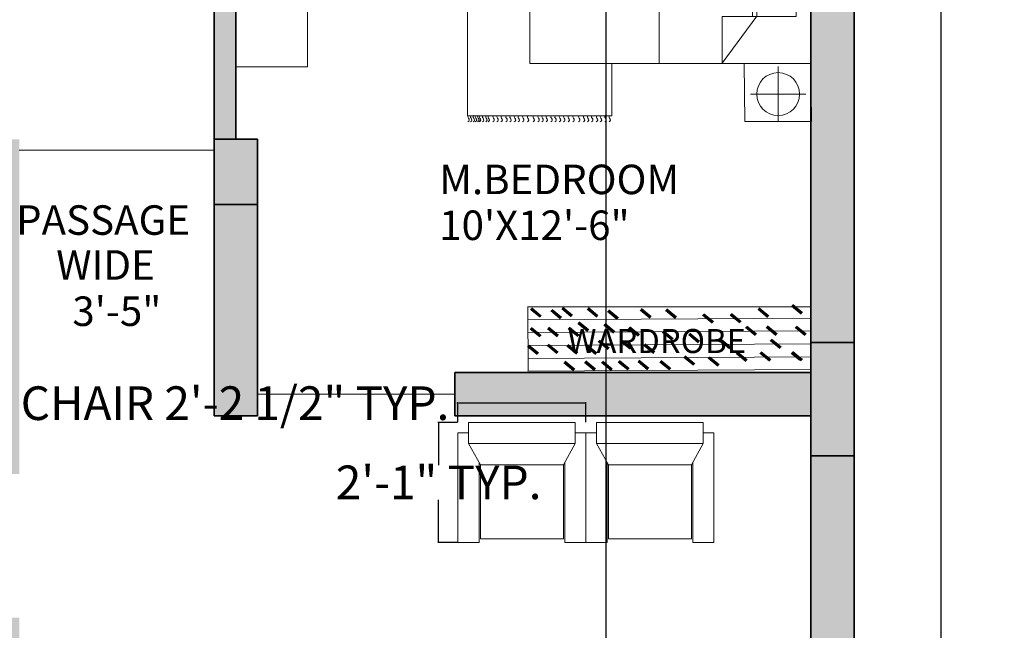
# Model space of a CAD drawing. Units: inches. Extents: x -17 to 892, y -721 to 172.
# Tile 5 of 11: x 174 to 378, y -209 to -82. Entities that reach past the tile are written whole.
import ezdxf

# ---------------------------------------------------------------- set-up
doc = ezdxf.new("R2010")
doc.units = ezdxf.units.IN
doc.header["$MEASUREMENT"] = 0
doc.layers.get('0').update_dxf_attribs({"color": 14})
for name, color, linetype, lineweight in [('A-ANNO-DIMS', 2, 'Continuous', 18), ('A-ANNO-TEXT', 7, 'Continuous', 18), ('A-AREA-IDEN', 7, 'Continuous', 18), ('A-COLS', 252, 'Continuous', 35), ('A-FLOR-CASE', 252, 'Continuous', 18), ('A-FURN-PATT', 252, 'Continuous', 9), ('A-WALL-PATT', 14, 'Continuous', 13), ('doors', 4, 'Continuous', 18), ('furniture', 252, 'Continuous', 18), ('walls', 252, 'Continuous', 35)]:
    doc.layers.add(name, color=color, linetype=linetype, lineweight=lineweight)
doc.layers.add('A-COLS-PATT', color=254, linetype='Continuous', lineweight=13, true_color=0xd7ebd2)
doc.styles.get("Standard").update_dxf_attribs({"font": 'arial.ttf'})
doc.dimstyles.get("Standard").update_dxf_attribs({"dimtxt": 7, "dimasz": 0.18, "dimexe": 0.18, "dimexo": 0.0625, "dimgap": 0.09, "dimtad": 0, "dimtih": 1, "dimtoh": 1, "dimzin": 0, "dimdsep": 46, "dimlunit": 3, "dimtxsty": 'Standard', "dimcen": 0.09, "dimadec": 0, "dimazin": 0, "dimtfac": 1, "dimtofl": 0, "dimtmove": 0, "dimatfit": 3, "dimfxl": 1, "dimtolj": 1, "dimtzin": 0, "dimarcsym": 0})

# ---------------------------------------------------------------- blocks, each defined once
blk = doc.blocks.new('CARPET')
at = {"layer": 'furniture'}
for p, q in [((-51.53, -98.11), (-51.53, -55.12)), ((-51.53, -55.12), (-41.27, -55.12)), ((36, -55.12), (51.55, -55.12)), ((51.55, -55.12), (51.55, -98.11)), ((51.55, -98.11), (-51.53, -98.11))]:
    blk.add_line(p, q, dxfattribs=at)
for points, knots in [([(-53.37, -55.99), (-53.22, -55.8), (-52.9, -55.41), (-52.34, -55.8), (-51.89, -56.08), (-51.65, -55.91), (-51.53, -55.83)], [0, 0, 0, 0, 0.653278, 1.290138, 1.740457, 2.114451, 2.114451, 2.114451, 2.114451]), ([(53.37, -55.99), (53.22, -55.8), (52.9, -55.41), (52.34, -55.8), (51.89, -56.08), (51.65, -55.91), (51.53, -55.83)], [0, 0, 0, 0, 0.653278, 1.290138, 1.740457, 2.114451, 2.114451, 2.114451, 2.114451]), ([(-53.37, -57.26), (-53.22, -57.07), (-52.9, -56.67), (-52.34, -57.07), (-51.89, -57.35), (-51.65, -57.17), (-51.53, -57.1)], [0, 0, 0, 0, 0.653278, 1.290138, 1.740457, 2.114451, 2.114451, 2.114451, 2.114451]), ([(-53.37, -58.59), (-53.22, -58.4), (-52.9, -58.01), (-52.34, -58.4), (-51.89, -58.68), (-51.65, -58.5), (-51.53, -58.43)], [0, 0, 0, 0, 0.653278, 1.290138, 1.740457, 2.114451, 2.114451, 2.114451, 2.114451]), ([(53.37, -57.26), (53.22, -57.07), (52.9, -56.67), (52.34, -57.07), (51.89, -57.35), (51.65, -57.17), (51.53, -57.1)], [0, 0, 0, 0, 0.653278, 1.290138, 1.740457, 2.114451, 2.114451, 2.114451, 2.114451]), ([(53.37, -58.59), (53.22, -58.4), (52.9, -58.01), (52.34, -58.4), (51.89, -58.68), (51.65, -58.5), (51.53, -58.43)], [0, 0, 0, 0, 0.653278, 1.290138, 1.740457, 2.114451, 2.114451, 2.114451, 2.114451]), ([(-53.37, -59.78), (-53.22, -59.58), (-52.9, -59.19), (-52.34, -59.58), (-51.89, -59.86), (-51.65, -59.69), (-51.53, -59.61)], [0, 0, 0, 0, 0.653278, 1.290138, 1.740457, 2.114451, 2.114451, 2.114451, 2.114451]), ([(-53.37, -61.22), (-53.22, -61.02), (-52.9, -60.63), (-52.34, -61.02), (-51.89, -61.3), (-51.65, -61.13), (-51.53, -61.05)], [0, 0, 0, 0, 0.653278, 1.290138, 1.740457, 2.114451, 2.114451, 2.114451, 2.114451]), ([(53.37, -59.78), (53.22, -59.58), (52.9, -59.19), (52.34, -59.58), (51.89, -59.86), (51.65, -59.69), (51.53, -59.61)], [0, 0, 0, 0, 0.653278, 1.290138, 1.740457, 2.114451, 2.114451, 2.114451, 2.114451]), ([(53.37, -61.22), (53.22, -61.02), (52.9, -60.63), (52.34, -61.02), (51.89, -61.3), (51.65, -61.13), (51.53, -61.05)], [0, 0, 0, 0, 0.653278, 1.290138, 1.740457, 2.114451, 2.114451, 2.114451, 2.114451]), ([(-53.37, -62.44), (-53.22, -62.25), (-52.9, -61.86), (-52.34, -62.25), (-51.89, -62.53), (-51.65, -62.36), (-51.53, -62.28)], [0, 0, 0, 0, 0.653278, 1.290138, 1.740457, 2.114451, 2.114451, 2.114451, 2.114451]), ([(-53.37, -63.63), (-53.22, -63.43), (-52.9, -63.04), (-52.34, -63.43), (-51.89, -63.72), (-51.65, -63.54), (-51.53, -63.46)], [0, 0, 0, 0, 0.653278, 1.290138, 1.740457, 2.114451, 2.114451, 2.114451, 2.114451]), ([(53.37, -62.44), (53.22, -62.25), (52.9, -61.86), (52.34, -62.25), (51.89, -62.53), (51.65, -62.36), (51.53, -62.28)], [0, 0, 0, 0, 0.653278, 1.290138, 1.740457, 2.114451, 2.114451, 2.114451, 2.114451]), ([(53.37, -63.63), (53.22, -63.43), (52.9, -63.04), (52.34, -63.43), (51.89, -63.72), (51.65, -63.54), (51.53, -63.46)], [0, 0, 0, 0, 0.653278, 1.290138, 1.740457, 2.114451, 2.114451, 2.114451, 2.114451]), ([(-53.37, -65.07), (-53.22, -64.87), (-52.9, -64.48), (-52.34, -64.87), (-51.89, -65.15), (-51.65, -64.98), (-51.53, -64.9)], [0, 0, 0, 0, 0.653278, 1.290138, 1.740457, 2.114451, 2.114451, 2.114451, 2.114451]), ([(-53.37, -66.76), (-53.22, -66.56), (-52.9, -66.17), (-52.34, -66.56), (-51.89, -66.84), (-51.65, -66.67), (-51.53, -66.59)], [0, 0, 0, 0, 0.653278, 1.290138, 1.740457, 2.114451, 2.114451, 2.114451, 2.114451]), ([(53.37, -65.07), (53.22, -64.87), (52.9, -64.48), (52.34, -64.87), (51.89, -65.15), (51.65, -64.98), (51.53, -64.9)], [0, 0, 0, 0, 0.653278, 1.290138, 1.740457, 2.114451, 2.114451, 2.114451, 2.114451]), ([(53.37, -66.76), (53.22, -66.56), (52.9, -66.17), (52.34, -66.56), (51.89, -66.84), (51.65, -66.67), (51.53, -66.59)], [0, 0, 0, 0, 0.653278, 1.290138, 1.740457, 2.114451, 2.114451, 2.114451, 2.114451]), ([(-53.37, -68.2), (-53.22, -68), (-52.9, -67.61), (-52.34, -68), (-51.89, -68.28), (-51.65, -68.11), (-51.53, -68.03)], [0, 0, 0, 0, 0.653278, 1.290138, 1.740457, 2.114451, 2.114451, 2.114451, 2.114451]), ([(-53.37, -69.53), (-53.22, -69.33), (-52.9, -68.94), (-52.34, -69.33), (-51.89, -69.61), (-51.65, -69.44), (-51.53, -69.36)], [0, 0, 0, 0, 0.653278, 1.290138, 1.740457, 2.114451, 2.114451, 2.114451, 2.114451]), ([(53.37, -68.2), (53.22, -68), (52.9, -67.61), (52.34, -68), (51.89, -68.28), (51.65, -68.11), (51.53, -68.03)], [0, 0, 0, 0, 0.653278, 1.290138, 1.740457, 2.114451, 2.114451, 2.114451, 2.114451]), ([(53.37, -69.53), (53.22, -69.33), (52.9, -68.94), (52.34, -69.33), (51.89, -69.61), (51.65, -69.44), (51.53, -69.36)], [0, 0, 0, 0, 0.653278, 1.290138, 1.740457, 2.114451, 2.114451, 2.114451, 2.114451]), ([(-53.37, -70.79), (-53.22, -70.6), (-52.9, -70.21), (-52.34, -70.6), (-51.89, -70.88), (-51.65, -70.7), (-51.53, -70.63)], [0, 0, 0, 0, 0.653278, 1.290138, 1.740457, 2.114451, 2.114451, 2.114451, 2.114451]), ([(-53.37, -72.12), (-53.22, -71.93), (-52.9, -71.54), (-52.34, -71.93), (-51.89, -72.21), (-51.65, -72.04), (-51.53, -71.96)], [0, 0, 0, 0, 0.653278, 1.290138, 1.740457, 2.114451, 2.114451, 2.114451, 2.114451]), ([(-53.37, -73.31), (-53.22, -73.11), (-52.9, -72.72), (-52.34, -73.11), (-51.89, -73.4), (-51.65, -73.22), (-51.53, -73.14)], [0, 0, 0, 0, 0.653278, 1.290138, 1.740457, 2.114451, 2.114451, 2.114451, 2.114451]), ([(53.37, -70.79), (53.22, -70.6), (52.9, -70.21), (52.34, -70.6), (51.89, -70.88), (51.65, -70.7), (51.53, -70.63)], [0, 0, 0, 0, 0.653278, 1.290138, 1.740457, 2.114451, 2.114451, 2.114451, 2.114451]), ([(53.37, -72.12), (53.22, -71.93), (52.9, -71.54), (52.34, -71.93), (51.89, -72.21), (51.65, -72.04), (51.53, -71.96)], [0, 0, 0, 0, 0.653278, 1.290138, 1.740457, 2.114451, 2.114451, 2.114451, 2.114451]), ([(53.37, -73.31), (53.22, -73.11), (52.9, -72.72), (52.34, -73.11), (51.89, -73.4), (51.65, -73.22), (51.53, -73.14)], [0, 0, 0, 0, 0.653278, 1.290138, 1.740457, 2.114451, 2.114451, 2.114451, 2.114451]), ([(-53.37, -74.75), (-53.22, -74.55), (-52.9, -74.16), (-52.34, -74.55), (-51.89, -74.83), (-51.65, -74.66), (-51.53, -74.58)], [0, 0, 0, 0, 0.653278, 1.290138, 1.740457, 2.114451, 2.114451, 2.114451, 2.114451]), ([(-53.37, -75.98), (-53.22, -75.78), (-52.9, -75.39), (-52.34, -75.78), (-51.89, -76.06), (-51.65, -75.89), (-51.53, -75.81)], [0, 0, 0, 0, 0.653278, 1.290138, 1.740457, 2.114451, 2.114451, 2.114451, 2.114451]), ([(53.37, -74.75), (53.22, -74.55), (52.9, -74.16), (52.34, -74.55), (51.89, -74.83), (51.65, -74.66), (51.53, -74.58)], [0, 0, 0, 0, 0.653278, 1.290138, 1.740457, 2.114451, 2.114451, 2.114451, 2.114451]), ([(53.37, -75.98), (53.22, -75.78), (52.9, -75.39), (52.34, -75.78), (51.89, -76.06), (51.65, -75.89), (51.53, -75.81)], [0, 0, 0, 0, 0.653278, 1.290138, 1.740457, 2.114451, 2.114451, 2.114451, 2.114451]), ([(-53.37, -77.16), (-53.22, -76.96), (-52.9, -76.57), (-52.34, -76.96), (-51.89, -77.25), (-51.65, -77.07), (-51.53, -76.99)], [0, 0, 0, 0, 0.653278, 1.290138, 1.740457, 2.114451, 2.114451, 2.114451, 2.114451]), ([(-53.37, -78.6), (-53.22, -78.4), (-52.9, -78.01), (-52.34, -78.4), (-51.89, -78.68), (-51.65, -78.51), (-51.53, -78.43)], [0, 0, 0, 0, 0.653278, 1.290138, 1.740457, 2.114451, 2.114451, 2.114451, 2.114451]), ([(53.37, -77.16), (53.22, -76.96), (52.9, -76.57), (52.34, -76.96), (51.89, -77.25), (51.65, -77.07), (51.53, -76.99)], [0, 0, 0, 0, 0.653278, 1.290138, 1.740457, 2.114451, 2.114451, 2.114451, 2.114451]), ([(53.37, -78.6), (53.22, -78.4), (52.9, -78.01), (52.34, -78.4), (51.89, -78.68), (51.65, -78.51), (51.53, -78.43)], [0, 0, 0, 0, 0.653278, 1.290138, 1.740457, 2.114451, 2.114451, 2.114451, 2.114451]), ([(-53.37, -80.29), (-53.22, -80.09), (-52.9, -79.7), (-52.34, -80.09), (-51.89, -80.37), (-51.65, -80.2), (-51.53, -80.12)], [0, 0, 0, 0, 0.653278, 1.290138, 1.740457, 2.114451, 2.114451, 2.114451, 2.114451]), ([(-53.37, -81.73), (-53.22, -81.53), (-52.9, -81.14), (-52.34, -81.53), (-51.89, -81.81), (-51.65, -81.64), (-51.53, -81.56)], [0, 0, 0, 0, 0.653278, 1.290138, 1.740457, 2.114451, 2.114451, 2.114451, 2.114451]), ([(53.37, -80.29), (53.22, -80.09), (52.9, -79.7), (52.34, -80.09), (51.89, -80.37), (51.65, -80.2), (51.53, -80.12)], [0, 0, 0, 0, 0.653278, 1.290138, 1.740457, 2.114451, 2.114451, 2.114451, 2.114451]), ([(53.37, -81.73), (53.22, -81.53), (52.9, -81.14), (52.34, -81.53), (51.89, -81.81), (51.65, -81.64), (51.53, -81.56)], [0, 0, 0, 0, 0.653278, 1.290138, 1.740457, 2.114451, 2.114451, 2.114451, 2.114451]), ([(-53.37, -83.06), (-53.22, -82.86), (-52.9, -82.47), (-52.34, -82.86), (-51.89, -83.14), (-51.65, -82.97), (-51.53, -82.89)], [0, 0, 0, 0, 0.653278, 1.290138, 1.740457, 2.114451, 2.114451, 2.114451, 2.114451]), ([(-53.37, -84.18), (-53.22, -83.99), (-52.9, -83.6), (-52.34, -83.99), (-51.89, -84.27), (-51.65, -84.09), (-51.53, -84.02)], [0, 0, 0, 0, 0.653278, 1.290138, 1.740457, 2.114451, 2.114451, 2.114451, 2.114451]), ([(53.37, -83.06), (53.22, -82.86), (52.9, -82.47), (52.34, -82.86), (51.89, -83.14), (51.65, -82.97), (51.53, -82.89)], [0, 0, 0, 0, 0.653278, 1.290138, 1.740457, 2.114451, 2.114451, 2.114451, 2.114451]), ([(53.37, -84.18), (53.22, -83.99), (52.9, -83.6), (52.34, -83.99), (51.89, -84.27), (51.65, -84.09), (51.53, -84.02)], [0, 0, 0, 0, 0.653278, 1.290138, 1.740457, 2.114451, 2.114451, 2.114451, 2.114451]), ([(-53.37, -85.51), (-53.22, -85.32), (-52.9, -84.93), (-52.34, -85.32), (-51.89, -85.6), (-51.65, -85.42), (-51.53, -85.35)], [0, 0, 0, 0, 0.653278, 1.290138, 1.740457, 2.114451, 2.114451, 2.114451, 2.114451]), ([(-53.37, -86.7), (-53.22, -86.5), (-52.9, -86.11), (-52.34, -86.5), (-51.89, -86.78), (-51.65, -86.61), (-51.53, -86.53)], [0, 0, 0, 0, 0.653278, 1.290138, 1.740457, 2.114451, 2.114451, 2.114451, 2.114451]), ([(-53.37, -88.14), (-53.22, -87.94), (-52.9, -87.55), (-52.34, -87.94), (-51.89, -88.22), (-51.65, -88.05), (-51.53, -87.97)], [0, 0, 0, 0, 0.653278, 1.290138, 1.740457, 2.114451, 2.114451, 2.114451, 2.114451]), ([(53.37, -85.51), (53.22, -85.32), (52.9, -84.93), (52.34, -85.32), (51.89, -85.6), (51.65, -85.42), (51.53, -85.35)], [0, 0, 0, 0, 0.653278, 1.290138, 1.740457, 2.114451, 2.114451, 2.114451, 2.114451]), ([(53.37, -86.7), (53.22, -86.5), (52.9, -86.11), (52.34, -86.5), (51.89, -86.78), (51.65, -86.61), (51.53, -86.53)], [0, 0, 0, 0, 0.653278, 1.290138, 1.740457, 2.114451, 2.114451, 2.114451, 2.114451]), ([(53.37, -88.14), (53.22, -87.94), (52.9, -87.55), (52.34, -87.94), (51.89, -88.22), (51.65, -88.05), (51.53, -87.97)], [0, 0, 0, 0, 0.653278, 1.290138, 1.740457, 2.114451, 2.114451, 2.114451, 2.114451]), ([(-53.37, -89.36), (-53.22, -89.17), (-52.9, -88.78), (-52.34, -89.17), (-51.89, -89.45), (-51.65, -89.28), (-51.53, -89.2)], [0, 0, 0, 0, 0.653278, 1.290138, 1.740457, 2.114451, 2.114451, 2.114451, 2.114451]), ([(-53.37, -90.55), (-53.22, -90.35), (-52.9, -89.96), (-52.34, -90.35), (-51.89, -90.64), (-51.65, -90.46), (-51.53, -90.38)], [0, 0, 0, 0, 0.653278, 1.290138, 1.740457, 2.114451, 2.114451, 2.114451, 2.114451]), ([(53.37, -89.36), (53.22, -89.17), (52.9, -88.78), (52.34, -89.17), (51.89, -89.45), (51.65, -89.28), (51.53, -89.2)], [0, 0, 0, 0, 0.653278, 1.290138, 1.740457, 2.114451, 2.114451, 2.114451, 2.114451]), ([(53.37, -90.55), (53.22, -90.35), (52.9, -89.96), (52.34, -90.35), (51.9, -90.63), (51.66, -90.47), (51.55, -90.4)], [0, 0, 0, 0, 0.653278, 1.290138, 1.740457, 2.0926, 2.0926, 2.0926, 2.0926]), ([(-53.37, -91.99), (-53.22, -91.79), (-52.9, -91.4), (-52.34, -91.79), (-51.89, -92.07), (-51.65, -91.9), (-51.53, -91.82)], [0, 0, 0, 0, 0.653278, 1.290138, 1.740457, 2.114451, 2.114451, 2.114451, 2.114451]), ([(-53.37, -92.69), (-53.22, -92.48), (-52.9, -92.08), (-52.35, -92.49), (-51.89, -92.77), (-51.65, -92.6), (-51.53, -92.52)], [0, 0, 0, 0, 0.663904, 1.307406, 1.757725, 2.131719, 2.131719, 2.131719, 2.131719]), ([(-53.37, -93.61), (-53.22, -93.42), (-52.9, -93.03), (-52.34, -93.42), (-51.89, -93.7), (-51.65, -93.52), (-51.53, -93.45)], [0, 0, 0, 0, 0.653278, 1.290138, 1.740457, 2.114451, 2.114451, 2.114451, 2.114451]), ([(53.37, -91.99), (53.22, -91.79), (52.9, -91.4), (52.34, -91.79), (51.9, -92.07), (51.66, -91.91), (51.55, -91.83)], [0, 0, 0, 0, 0.653278, 1.290138, 1.740457, 2.0926, 2.0926, 2.0926, 2.0926]), ([(53.37, -92.69), (53.22, -92.49), (52.9, -92.09), (52.34, -92.49), (51.9, -92.77), (51.66, -92.61), (51.55, -92.53)], [0, 0, 0, 0, 0.656792, 1.295826, 1.746145, 2.098292, 2.098292, 2.098292, 2.098292]), ([(53.37, -93.66), (53.22, -93.46), (52.9, -93.07), (52.34, -93.46), (51.9, -93.74), (51.66, -93.58), (51.55, -93.5)], [0, 0, 0, 0, 0.653278, 1.290138, 1.740457, 2.0926, 2.0926, 2.0926, 2.0926]), ([(-53.37, -94.55), (-53.22, -94.35), (-52.9, -93.96), (-52.34, -94.35), (-51.89, -94.63), (-51.65, -94.46), (-51.53, -94.38)], [0, 0, 0, 0, 0.653278, 1.290138, 1.740457, 2.114451, 2.114451, 2.114451, 2.114451]), ([(-53.37, -95.05), (-53.22, -94.85), (-52.9, -94.46), (-52.34, -94.85), (-51.89, -95.14), (-51.65, -94.96), (-51.53, -94.88)], [0, 0, 0, 0, 0.653278, 1.290138, 1.740457, 2.114451, 2.114451, 2.114451, 2.114451]), ([(-53.37, -95.73), (-53.22, -95.54), (-52.9, -95.15), (-52.34, -95.54), (-51.89, -95.82), (-51.65, -95.65), (-51.53, -95.57)], [0, 0, 0, 0, 0.653278, 1.290138, 1.740457, 2.114451, 2.114451, 2.114451, 2.114451]), ([(-53.37, -96.38), (-53.22, -96.18), (-52.9, -95.79), (-52.34, -96.18), (-51.89, -96.47), (-51.65, -96.29), (-51.53, -96.21)], [0, 0, 0, 0, 0.653278, 1.290138, 1.740457, 2.114451, 2.114451, 2.114451, 2.114451]), ([(53.37, -95.78), (53.22, -95.58), (52.9, -95.19), (52.34, -95.58), (51.89, -95.86), (51.65, -95.69), (51.53, -95.61)], [0, 0, 0, 0, 0.653278, 1.290138, 1.740457, 2.114451, 2.114451, 2.114451, 2.114451]), ([(53.37, -96.43), (53.22, -96.23), (52.9, -95.84), (52.34, -96.23), (51.89, -96.51), (51.65, -96.34), (51.53, -96.26)], [0, 0, 0, 0, 0.653278, 1.290138, 1.740457, 2.114451, 2.114451, 2.114451, 2.114451]), ([(53.37, -94.59), (53.22, -94.4), (52.9, -94.01), (52.34, -94.4), (51.9, -94.68), (51.66, -94.51), (51.55, -94.44)], [0, 0, 0, 0, 0.653278, 1.290138, 1.740457, 2.0926, 2.0926, 2.0926, 2.0926]), ([(53.37, -95.1), (53.22, -94.9), (52.9, -94.51), (52.34, -94.9), (51.9, -95.18), (51.66, -95.02), (51.55, -94.94)], [0, 0, 0, 0, 0.653278, 1.290138, 1.740457, 2.0926, 2.0926, 2.0926, 2.0926]), ([(-53.37, -97.17), (-53.22, -96.98), (-52.9, -96.59), (-52.34, -96.98), (-51.89, -97.26), (-51.65, -97.08), (-51.53, -97.01)], [0, 0, 0, 0, 0.653278, 1.290138, 1.740457, 2.114451, 2.114451, 2.114451, 2.114451]), ([(-53.37, -97.99), (-53.22, -97.79), (-52.9, -97.4), (-52.34, -97.79), (-51.89, -98.08), (-51.65, -97.9), (-51.53, -97.82)], [0, 0, 0, 0, 0.653278, 1.290138, 1.740457, 2.114451, 2.114451, 2.114451, 2.114451]), ([(53.37, -97.22), (53.22, -97.02), (52.9, -96.63), (52.34, -97.02), (51.89, -97.3), (51.65, -97.13), (51.53, -97.05)], [0, 0, 0, 0, 0.653278, 1.290138, 1.740457, 2.114451, 2.114451, 2.114451, 2.114451]), ([(53.37, -97.99), (53.22, -97.79), (52.9, -97.4), (52.34, -97.79), (51.89, -98.08), (51.65, -97.9), (51.53, -97.82)], [0, 0, 0, 0, 0.653278, 1.290138, 1.740457, 2.114451, 2.114451, 2.114451, 2.114451])]:
    blk.add_open_spline(points, degree=3, knots=knots, dxfattribs=at)
blk = doc.blocks.new('A$C58D270C6')
at = {"layer": 'furniture'}
for p, q in [((9.09, 124.13), (9.09, 108.87)), ((1.46, 116.5), (16.73, 116.5)), ((14.97, 94.84), (24.62, 107.92)), ((24.62, 94.93), (24.62, 107.92)), ((42.08, 108), (42.08, 36)), ((14.97, 94.93), (24.62, 94.93)), ((14.97, 94.84), (14.97, 36)), ((16.22, 94.93), (16.22, 36)), ((9.25, 36), (9.25, 20.74)), ((1.62, 28.37), (16.88, 28.37))]:
    blk.add_line(p, q, dxfattribs=at)
for points in [[(18.5, 108), (18.34, 124.13), (-0.16, 124.13), (0, 108)], [(0, 108), (77.91, 108), (77.91, 36), (0, 36)], [(4.09, 94.93), (14.97, 94.93), (14.97, 73.83), (4.09, 73.83)], [(4.09, 65.23), (14.97, 65.23), (14.97, 44.13), (4.09, 44.13)], [(18.65, 19.87), (18.5, 36), (0, 36), (0.16, 19.87)]]:
    blk.add_lwpolyline(points, close=True, dxfattribs=at)
for centre in [(9.09, 116.5), (9.25, 28.37)]:
    blk.add_circle(centre, 5.95, dxfattribs=at)
at = {"layer": 'furniture', "xscale": 0.9312884925094044, "yscale": 0.9312884925094044, "zscale": 0.9312884925094044, "rotation": 90}
blk.add_blockref('CARPET', (3.79, 74.47), dxfattribs=at)
blk = doc.blocks.new('FABRIC SOFA 1S')
at = {"layer": 'furniture'}
for p, q in [((3, 18.12), (34, 18.12)), ((3, 15.12), (3, 18.12)), ((34, 12.12), (34, 18.12)), ((0, -15.12), (0, 15.12)), ((6, 15.12), (0, 15.12)), ((6, -15.12), (6, 15.12)), ((12, 11.75), (6, 15.12)), ((11.33, 12.12), (34, 12.12)), ((6, -15.12), (12, -11.75)), ((11.33, -12.12), (34, -12.12)), ((34, -12.12), (34, -18.12)), ((6, -15.12), (0, -15.12)), ((3, -18.12), (3, -15.12)), ((3, -18.12), (34, -18.12))]:
    blk.add_line(p, q, dxfattribs=at)
blk.add_lwpolyline([(12, -11.75), (12, 11.75), (33, 11.75), (33, -11.75)], close=True, dxfattribs=at)
blk = doc.blocks.new('*D16')
at = {"layer": 'A-ANNO-DIMS', "color": 0, "lineweight": -2, "transparency": 16777216}
for p, q in [((364.49, 89.9), (365.24, 89.9)), ((365.06, 89.72), (365.06, -263.08)), ((365.06, -623.21), (365.06, -270.41)), ((364.49, -623.39), (365.24, -623.39))]:
    blk.add_line(p, q, dxfattribs=at)
at = {"layer": 'A-ANNO-DIMS', "color": 0, "lineweight": 100, "transparency": 16777216}
for points in [[(365.03, 89.72), (365.09, 89.72), (365.06, 89.9)], [(365.03, -623.21), (365.09, -623.21), (365.06, -623.39)]]:
    blk.add_solid(points, dxfattribs=at)
at = {"layer": 'Defpoints', "color": 0, "lineweight": 100, "transparency": 16777216}
for p in [(364.43, 89.9), (364.43, -623.39), (365.06, -623.39)]:
    blk.add_point(p, dxfattribs=at)
at = {"layer": 'A-ANNO-DIMS', "color": 0, "transparency": 16777216, "insert": (365.06, -266.74), "char_height": 7, "attachment_point": 5}
blk.add_mtext('\\A1;57\'-1"', dxfattribs=at)
blk = doc.blocks.new('WARDROBE-59-PLAN')
for p, q in [((0, 13.37), (58.88, 13.37)), ((0.05, 13.37), (0.13, 0)), ((58.95, 0.34), (58.88, 13.71)), ((0.02, 10.69), (58.89, 11.04)), ((0.03, 8.02), (58.91, 8.36)), ((0.05, 5.35), (58.92, 5.69)), ((0.06, 2.67), (58.94, 3.02)), ((0.08, 0), (58.95, 0.34))]:
    blk.add_line(p, q)
blk = doc.blocks.new('MEDIA-CONSOLE')
for p, q in [((14.9, 64.44), (0, 64.44)), ((14.9, 0), (14.9, 64.44)), ((0, 0), (14.9, 0))]:
    blk.add_line(p, q)
blk = doc.blocks.new('*D28')
at = {"layer": 'A-ANNO-DIMS', "color": 0, "lineweight": -2, "transparency": 16777216}
for p, q in [((264.71, -161.27), (264.53, -161.27)), ((264.71, -165.2), (264.71, -161.09)), ((291.14, -161.27), (264.89, -161.27)), ((291.32, -165.2), (291.32, -161.09))]:
    blk.add_line(p, q, dxfattribs=at)
at = {"layer": 'A-ANNO-DIMS', "color": 0, "lineweight": 100, "transparency": 16777216}
for points in [[(264.89, -161.24), (264.89, -161.3), (264.71, -161.27)], [(291.14, -161.24), (291.14, -161.3), (291.32, -161.27)]]:
    blk.add_solid(points, dxfattribs=at)
at = {"layer": 'Defpoints', "color": 0, "lineweight": 100, "transparency": 16777216}
for p in [(264.71, -161.27), (264.71, -165.26), (291.32, -165.26)]:
    blk.add_point(p, dxfattribs=at)
at = {"layer": 'A-ANNO-DIMS', "color": 0, "transparency": 16777216, "insert": (218.42, -161.27), "char_height": 7, "attachment_point": 5}
blk.add_mtext('\\A1;CHAIR 2\'-2 1/2" TYP.', dxfattribs=at)
blk = doc.blocks.new('*D29')
at = {"layer": 'A-ANNO-DIMS', "color": 0, "lineweight": -2, "transparency": 16777216}
for p, q in [((264.65, -165.26), (260.54, -165.26)), ((260.72, -165.44), (260.72, -174.13)), ((260.72, -190.04), (260.72, -181.35)), ((264.65, -190.22), (260.54, -190.22))]:
    blk.add_line(p, q, dxfattribs=at)
at = {"layer": 'A-ANNO-DIMS', "color": 0, "lineweight": 100, "transparency": 16777216}
for points in [[(260.69, -165.44), (260.75, -165.44), (260.72, -165.26)], [(260.69, -190.04), (260.75, -190.04), (260.72, -190.22)]]:
    blk.add_solid(points, dxfattribs=at)
at = {"layer": 'Defpoints', "color": 0, "lineweight": 100, "transparency": 16777216}
for p in [(264.71, -165.26), (260.72, -190.22), (264.71, -190.22)]:
    blk.add_point(p, dxfattribs=at)
at = {"layer": 'A-ANNO-DIMS', "color": 0, "transparency": 16777216, "insert": (260.72, -177.74), "char_height": 7, "attachment_point": 5}
blk.add_mtext('\\A1;2\'-1" TYP.', dxfattribs=at)
blk = doc.blocks.new('*D63')
at = {"layer": 'A-ANNO-DIMS', "color": 0, "lineweight": -2, "transparency": 16777216}
for p, q in [((295.55, -619.99), (295.55, 161.84)), ((295.73, 161.66), (299.27, 161.66)), ((337.9, 161.66), (334.36, 161.66)), ((338.08, -619.99), (338.08, 161.84))]:
    blk.add_line(p, q, dxfattribs=at)
at = {"layer": 'A-ANNO-DIMS', "color": 0, "lineweight": 100, "transparency": 16777216}
for points in [[(295.73, 161.69), (295.73, 161.63), (295.55, 161.66)], [(337.9, 161.69), (337.9, 161.63), (338.08, 161.66)]]:
    blk.add_solid(points, dxfattribs=at)
at = {"layer": 'Defpoints', "color": 0, "lineweight": 100, "transparency": 16777216}
for p in [(338.08, 161.66), (295.55, -620.06), (338.08, -620.06)]:
    blk.add_point(p, dxfattribs=at)
at = {"layer": 'A-ANNO-DIMS', "color": 0, "transparency": 16777216, "insert": (316.82, 161.66), "char_height": 7, "attachment_point": 5}
blk.add_mtext('\\A1;3\'-6 1/2"', dxfattribs=at)

msp = doc.modelspace()

# ---------------------------------------------------------------- hatches: boundary and pattern name
at = {"layer": 'A-COLS-PATT'}
h = msp.add_hatch(color=256, dxfattribs=at)
h.dxf.hatch_style = 1
h.paths.add_polyline_path([(92.084, 61.611), (83.084, 61.611), (83.084, 43.692), (92.084, 43.692)])
h.paths.add_polyline_path([(347.084, 61.611), (338.084, 61.611), (338.084, 43.692), (347.084, 43.692)])
h.paths.add_polyline_path([(222.053, 61.611), (209.95, 61.611), (209.95, 52.611), (222.053, 52.611)])
h.paths.add_polyline_path([(284.798, 61.611), (274.584, 61.611), (274.584, 52.611), (284.798, 52.611)])
h.paths.add_polyline_path([(223.084, -106.389), (214.084, -106.389), (214.084, -119.959), (223.084, -119.959)])
h.paths.add_polyline_path([(347.084, -148.653), (338.084, -148.653), (338.084, -172.24), (347.084, -172.24)])
h.paths.add_polyline_path([(92.084, -102.402), (83.084, -102.402), (83.084, -119.959), (92.084, -119.959)])
h.paths.add_polyline_path([(92.084, -205.889), (83.084, -205.889), (83.084, -216.319), (92.084, -216.319)])
h.paths.add_polyline_path([(347.084, -349.073), (338.084, -349.073), (338.084, -372.66), (347.084, -372.66)])
h.paths.add_polyline_path([(347.084, -610.134), (338.084, -610.134), (338.084, -614.389), (338.084, -623.342), (347.084, -623.342)])
h.paths.add_polyline_path([(221.166, -610.357), (214.084, -610.357), (214.084, -623.389), (219.084, -623.389), (221.166, -623.389), (221.166, -621.723)])
h.paths.add_polyline_path([(90.166, -610.357), (83.084, -610.357), (83.084, -623.389), (90.166, -623.389)])
h.paths.add_polyline_path([(223.084, -401.64), (214.084, -401.64), (214.084, -410.389), (223.084, -410.389)])
h.paths.add_polyline_path([(223.084, -356.889), (214.084, -356.889), (214.084, -369.273), (223.084, -369.273)])
h.paths.add_polyline_path([(92.084, -398.492), (83.084, -398.492), (83.084, -410.389), (92.084, -410.389)])
h.paths.add_polyline_path([(92.084, -348.918), (83.084, -348.918), (83.084, -360.706), (92.084, -360.706)])
at = {"layer": 'A-FURN-PATT'}
h = msp.add_hatch(dxfattribs=at)
h.set_pattern_fill('ANSI31', color=256, scale=0.8475126, angle=95.46701, style=0)
h.paths.add_polyline_path([(279.153, -149.533), (281.149, -151.181), (281.487, -150.772), (279.49, -149.124)])
h.paths.add_polyline_path([(286.703, -152.935), (288.7, -154.583), (289.037, -154.174), (287.04, -152.526)], flags=0)
h.paths.add_polyline_path([(283.213, -149.381), (285.21, -151.029), (285.547, -150.621), (283.551, -148.973)], flags=0)
h.paths.add_polyline_path([(279.724, -145.89), (281.721, -147.538), (282.059, -147.13), (280.062, -145.482)], flags=0)
h.paths.add_polyline_path([(290.968, -152.88), (292.965, -154.528), (293.302, -154.119), (291.305, -152.471)], flags=0)
h.paths.add_polyline_path([(287.358, -149.43), (289.355, -151.078), (289.692, -150.67), (287.695, -149.022)], flags=0)
h.paths.add_polyline_path([(283.299, -145.869), (285.296, -147.517), (285.633, -147.109), (283.636, -145.461)], flags=0)
h.paths.add_polyline_path([(279.726, -141.84), (281.723, -143.488), (282.061, -143.08), (280.064, -141.432)], flags=0)
h.paths.add_polyline_path([(294.528, -152.858), (296.524, -154.506), (296.862, -154.098), (294.865, -152.45)], flags=0)
h.paths.add_polyline_path([(291.286, -149.529), (293.282, -151.177), (293.62, -150.769), (291.623, -149.121)], flags=0)
h.paths.add_polyline_path([(287.593, -145.844), (289.59, -147.492), (289.927, -147.084), (287.93, -145.435)], flags=0)
h.paths.add_polyline_path([(283.97, -142.139), (285.967, -143.787), (286.304, -143.378), (284.307, -141.73)], flags=0)
h.paths.add_polyline_path([(298.037, -152.713), (300.033, -154.361), (300.371, -153.952), (298.374, -152.304)], flags=0)
h.paths.add_polyline_path([(293.892, -148.48), (295.889, -150.128), (296.226, -149.72), (294.229, -148.072)], flags=0)
h.paths.add_polyline_path([(289.587, -144.76), (291.584, -146.408), (291.921, -145.999), (289.924, -144.351)], flags=0)
h.paths.add_polyline_path([(286.225, -141.718), (288.221, -143.366), (288.559, -142.957), (286.562, -141.309)], flags=0)
h.paths.add_polyline_path([(302.094, -152.725), (304.091, -154.373), (304.428, -153.964), (302.431, -152.316)], flags=0)
h.paths.add_polyline_path([(298.472, -148.454), (300.469, -150.102), (300.806, -149.693), (298.809, -148.045)], flags=0)
h.paths.add_polyline_path([(295.007, -145.114), (297.004, -146.762), (297.341, -146.353), (295.344, -144.705)], flags=0)
h.paths.add_polyline_path([(291.554, -141.738), (293.551, -143.386), (293.888, -142.978), (291.891, -141.33)], flags=0)
h.paths.add_polyline_path([(306.668, -152.777), (308.665, -154.425), (309.002, -154.016), (307.005, -152.368)], flags=0)
h.paths.add_polyline_path([(303.337, -149.278), (305.334, -150.926), (305.671, -150.518), (303.674, -148.87)], flags=0)
h.paths.add_polyline_path([(300.129, -145.771), (302.126, -147.419), (302.463, -147.01), (300.466, -145.362)], flags=0)
h.paths.add_polyline_path([(295.776, -142.245), (297.773, -143.893), (298.11, -143.485), (296.113, -141.837)], flags=0)
h.paths.add_polyline_path([(311.658, -151.766), (313.655, -153.414), (313.992, -153.005), (311.995, -151.357)], flags=0)
h.paths.add_polyline_path([(307.172, -146.556), (309.169, -148.204), (309.506, -147.795), (307.51, -146.147)], flags=0)
h.paths.add_polyline_path([(302.609, -141.96), (304.606, -143.608), (304.943, -143.199), (302.946, -141.551)], flags=0)
h.paths.add_polyline_path([(316.686, -151.982), (318.683, -153.63), (319.02, -153.221), (317.023, -151.573)], flags=0)
h.paths.add_polyline_path([(312.612, -147.138), (314.608, -148.786), (314.946, -148.377), (312.949, -146.729)], flags=0)
h.paths.add_polyline_path([(307.841, -142.052), (309.838, -143.7), (310.175, -143.291), (308.178, -141.643)], flags=0)
h.paths.add_polyline_path([(322.487, -150.986), (324.484, -152.634), (324.821, -152.226), (322.824, -150.578)], flags=0)
h.paths.add_polyline_path([(319.125, -148.333), (321.122, -149.981), (321.459, -149.572), (319.463, -147.924)], flags=0)
h.paths.add_polyline_path([(315.539, -143.007), (317.536, -144.655), (317.873, -144.246), (315.877, -142.598)], flags=0)
h.paths.add_polyline_path([(321.29, -142.973), (323.286, -144.621), (323.624, -144.213), (321.627, -142.565)], flags=0)
h.paths.add_polyline_path([(329.58, -148.271), (331.577, -149.919), (331.914, -149.511), (329.917, -147.863)], flags=0)
h.paths.add_polyline_path([(324.442, -145.628), (326.439, -147.276), (326.776, -146.868), (324.779, -145.22)], flags=0)
h.paths.add_polyline_path([(327.4, -150.957), (329.397, -152.605), (329.734, -152.197), (327.738, -150.549)], flags=0)
h.paths.add_polyline_path([(333.987, -150.919), (335.984, -152.567), (336.321, -152.158), (334.324, -150.51)], flags=0)
h.paths.add_polyline_path([(334.792, -145.567), (336.789, -147.216), (337.126, -146.807), (335.129, -145.159)], flags=0)
h.paths.add_polyline_path([(328.728, -145.603), (330.725, -147.251), (331.062, -146.842), (329.065, -145.194)], flags=0)
h.paths.add_polyline_path([(334.029, -141.118), (336.026, -142.766), (336.363, -142.357), (334.366, -140.709)], flags=0)
h.paths.add_polyline_path([(327.032, -141.842), (329.028, -143.49), (329.366, -143.082), (327.369, -141.434)], flags=0)
at = {"layer": 'A-WALL-PATT'}
h = msp.add_hatch(color=256, dxfattribs=at)
h.dxf.hatch_style = 1
h.paths.add_polyline_path([(111.26, 61.611), (92.084, 61.611), (92.084, 52.611), (111.26, 52.611)])
h.paths.add_polyline_path([(209.95, 61.611), (179.154, 61.611), (179.154, 52.611), (209.95, 52.611)])
h.paths.add_polyline_path([(338.084, 61.611), (284.798, 61.611), (284.798, 52.611), (338.084, 52.611)])
h.paths.add_polyline_path([(279.084, 23.861), (274.584, 23.861), (274.584, -0.389), (279.084, -0.389)])
h.paths.add_polyline_path([(279.084, 52.611), (274.584, 52.611), (274.584, 46.881), (276.834, 46.881), (279.084, 46.881)])
h.paths.add_polyline_path([(279.084, -0.389), (274.584, -0.389), (274.584, -4.889), (279.084, -4.889)])
h.paths.add_polyline_path([(304.22, -0.389), (279.084, -0.389), (279.084, -4.889), (304.22, -4.889)])
h.paths.add_polyline_path([(347.084, 43.692), (338.084, 43.692), (338.084, -148.653), (347.084, -148.653)])
h.paths.add_polyline_path([(338.084, -154.889), (264.103, -154.889), (264.103, -163.889), (338.084, -163.889)])
h.paths.add_polyline_path([(223.084, -119.959), (214.084, -119.959), (214.084, -163.889), (223.084, -163.889)])
h.paths.add_polyline_path([(218.584, 52.611), (214.084, 52.611), (214.084, -106.389), (218.584, -106.389)])
h.paths.add_polyline_path([(92.084, -8.943), (83.084, -8.943), (83.084, -49.69), (87.584, -49.69), (92.084, -49.69)])
h.paths.add_polyline_path([(92.084, 43.692), (83.084, 43.692), (83.084, 33.018), (87.584, 33.018), (92.084, 33.018)])
h.paths.add_polyline_path([(92.084, -91.651), (83.084, -91.651), (83.084, -102.402), (92.084, -102.402)])
h.paths.add_polyline_path([(92.084, -119.959), (83.084, -119.959), (83.084, -151.855), (87.584, -151.855), (92.084, -151.855)])
h.paths.add_polyline_path([(173.584, -108.639), (173.584, -106.389), (173.084, -106.389), (92.084, -106.389), (92.084, -110.889), (169.084, -110.889), (169.084, -176.029), (173.584, -176.029)])
h.paths.add_polyline_path([(92.084, -185.221), (83.084, -185.221), (83.084, -205.889), (92.084, -205.889)])
h.paths.add_polyline_path([(92.084, -216.319), (83.084, -216.319), (83.084, -259.015), (87.584, -259.015), (92.084, -259.015)])
h.paths.add_polyline_path([(173.584, -205.889), (92.084, -205.889), (92.084, -210.389), (169.084, -210.389), (169.084, -236.193), (173.584, -236.193)])
h.paths.add_polyline_path([(92.084, -300.976), (83.084, -300.976), (83.084, -348.918), (92.084, -348.918)])
h.paths.add_polyline_path([(87.584, -410.389), (83.084, -410.389), (83.084, -610.357), (87.584, -610.357)])
h.paths.add_polyline_path([(115.523, -614.389), (90.166, -614.389), (90.166, -623.389), (115.523, -623.389)])
h.paths.add_polyline_path([(214.084, -614.389), (174.149, -614.389), (174.149, -623.389), (214.084, -623.389)])
h.paths.add_polyline_path([(219.084, -410.389), (214.084, -410.389), (214.084, -610.357), (219.084, -610.357)])
h.paths.add_polyline_path([(347.084, -372.66), (338.084, -372.66), (338.084, -610.134), (347.084, -610.134)])
h.paths.add_polyline_path([(347.084, -172.24), (338.084, -172.24), (338.084, -349.073), (347.084, -349.073)])
h.paths.add_polyline_path([(338.084, -356.889), (317.618, -356.889), (317.618, -365.889), (338.084, -365.889)])
h.paths.add_polyline_path([(267.632, -356.889), (263.828, -356.889), (263.828, -365.889), (267.632, -365.889)])
h.paths.add_polyline_path([(223.084, -369.273), (214.084, -369.273), (214.084, -401.64), (223.084, -401.64)])

# ---------------------------------------------------------------- linework, layer by layer
at = {"layer": 'A-COLS'}
for p, q in [((214.084, -106.389), (223.084, -106.389)), ((214.084, -119.959), (223.084, -119.959)), ((338.084, -148.653), (347.084, -148.653)), ((338.084, -172.24), (347.084, -172.24))]:
    msp.add_line(p, q, dxfattribs=at)
at = {"layer": 'doors'}
for p, q in [((173.584, -108.639), (214.084, -108.639)), ((264.103, -159.389), (223.084, -159.389))]:
    msp.add_line(p, q, dxfattribs=at)
at = {"layer": 'walls'}
for p, q in [((338.084, 61.611), (338.084, -614.389)), ((347.084, 61.611), (347.084, -623.389)), ((214.084, -163.889), (214.084, 52.611)), ((218.584, -106.389), (218.584, 52.611)), ((223.084, -163.889), (223.084, -106.389)), ((264.103, -154.889), (338.084, -154.889)), ((264.103, -163.889), (264.103, -154.889)), ((223.084, -163.889), (214.084, -163.889)), ((264.103, -163.889), (338.084, -163.889))]:
    msp.add_line(p, q, dxfattribs=at)

# ---------------------------------------------------------------- block references
at = {"layer": 'A-FLOR-CASE'}
for name, p in [('MEDIA-CONSOLE', (218.584, -91.332)), ('WARDROBE-59-PLAN', (279.209, -154.62))]:
    msp.add_blockref(name, p, dxfattribs=at)
at = {"layer": 'furniture'}
for name, p, xscale, yscale, zscale, rotation in [('A$C58D270C6', (338.084, -9.622), 0.7500000390647866, 0.7500000390647866, 0.7500000390647866, 180), ('FABRIC SOFA 1S', (278.017, -165.263), -0.7339463821036302, 0.7339463821036302, 0.7339463821036302, 89.99999999999912), ('FABRIC SOFA 1S', (304.622, -165.263), -0.7339463821036302, 0.7339463821036302, 0.7339463821036302, 90)]:
    msp.add_blockref(name, p, dxfattribs=dict(at, xscale=xscale, yscale=yscale, zscale=zscale, rotation=rotation))

# ---------------------------------------------------------------- texts
at = {"layer": 'A-ANNO-TEXT'}
msp.add_text('WARDROBE', height=5, dxfattribs=at).set_placement((287.528, -150.845))
at = {"layer": 'A-AREA-IDEN'}
for s, p in [('M.BEDROOM', (260.851, -117.803)), ('PASSAGE', (172.922, -126.259)), ('10\'X12\'-6"', (260.851, -127.338)), ('WIDE', (181.26, -135.593)), ('3\'-5"', (184.618, -145.212))]:
    msp.add_text(s, height=6.1361, dxfattribs=at).set_placement(p)

# ---------------------------------------------------------------- dimensions: what is measured, and where the dimension line sits
at = {"layer": 'A-ANNO-DIMS'}
dim = msp.add_linear_dim(base=(338.084, 161.663), p1=(295.55, -620.057), p2=(338.084, -620.057), dimstyle='Standard', override={"dimdec": 1, "dimlfac": 1, "dimrnd": 0, "dimzin": 1, "dimdsep": 46, "dimlunit": 4, "dimfrac": 2}, dxfattribs=at)
dim.commit()
dim.dimension.update_dxf_attribs({"geometry": '*D63', "text_midpoint": (316.817, 161.663)})
for base, p1, p2, angle, text, override, picture, middle in [((365.057, -623.389), (364.432, 89.902), (364.432, -623.389), 90, '57\'-1"', {"dimclrd": 0, "dimclre": 0, "dimclrt": 0}, '*D16', (365.057, -266.744)), ((264.714, -161.272), (291.319, -165.263), (264.714, -165.263), 180, 'CHAIR <> TYP.', {"dimdec": 1, "dimlfac": 1, "dimrnd": 0, "dimzin": 1, "dimdsep": 46, "dimlunit": 4, "dimfrac": 2}, '*D28', (218.423, -161.272)), ((260.723, -190.217), (264.714, -165.263), (264.714, -190.217), 270, '<> TYP.', {"dimdec": 1, "dimlfac": 1, "dimrnd": 0, "dimzin": 1, "dimdsep": 46, "dimlunit": 4, "dimfrac": 2}, '*D29', (260.723, -177.74))]:
    dim = msp.add_linear_dim(base=base, p1=p1, p2=p2, angle=angle, text=text, dimstyle='Standard', override=override, dxfattribs=at)
    dim.commit()
    dim.dimension.update_dxf_attribs({"geometry": picture, "text_midpoint": middle})

doc.saveas('drawing.dxf')
